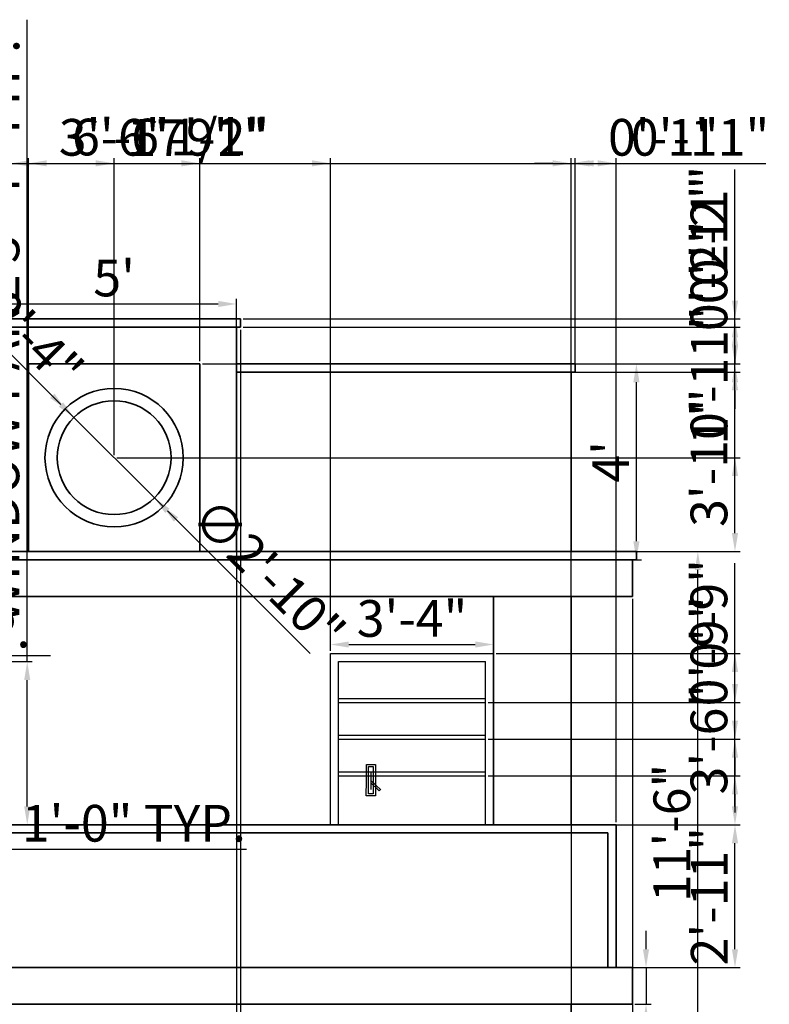
# Model space of a CAD drawing. Units: inches. Extents: x 3297 to 3846, y 520 to 959.
# Tile 5 of 5: x 3602 to 3786, y 717 to 959. Entities that reach past the tile are written whole.
import ezdxf

# ---------------------------------------------------------------- set-up
doc = ezdxf.new("R2010")
doc.units = ezdxf.units.IN
for name, color, linetype, lineweight in [('A-ANNO-DIMS', 2, 'Continuous', 18), ('A-DOOR', 4, 'Continuous', 25), ('A-ELEV', 7, 'Continuous', 35)]:
    doc.layers.add(name, color=color, linetype=linetype, lineweight=lineweight)
doc.styles.get("Standard").update_dxf_attribs({"font": 'arial.ttf'})
doc.dimstyles.new('ISO-25', dxfattribs={"dimtxt": 9, "dimasz": 4.5, "dimexe": 1.25, "dimexo": 0.625, "dimtad": 1, "dimdec": 0, "dimlunit": 3, "dimtxsty": 'Standard', "dimcen": 2.5, "dimadec": 0, "dimazin": 0, "dimtfac": 1, "dimtdec": 0, "dimtmove": 0, "dimatfit": 3, "dimfxl": 1, "dimarcsym": 0})

# ---------------------------------------------------------------- blocks, each defined once
blk = doc.blocks.new('*D2')
at = {"layer": 'A-ANNO-DIMS', "color": 0, "lineweight": -2, "transparency": 16777216}
for p, q in [((3752.69, 828.24), (3769.36, 828.24)), ((3768.11, 694.74), (3768.11, 823.74)), ((3752.69, 690.24), (3769.36, 690.24))]:
    blk.add_line(p, q, dxfattribs=at)
at = {"layer": 'A-ANNO-DIMS', "color": 0, "transparency": 16777216}
for points in [[(3767.36, 823.74), (3768.86, 823.74), (3768.11, 828.24)], [(3767.36, 694.74), (3768.86, 694.74), (3768.11, 690.24)]]:
    blk.add_solid(points, dxfattribs=at)
at = {"layer": 'Defpoints', "color": 0, "transparency": 16777216}
for p in [(3752.06, 828.24), (3768.11, 828.24), (3752.06, 690.24)]:
    blk.add_point(p, dxfattribs=at)
at = {"layer": 'A-ANNO-DIMS', "color": 0, "transparency": 16777216, "insert": (3762.89, 759.24), "char_height": 9, "attachment_point": 5, "rotation": 90}
blk.add_mtext('11\'-6"', dxfattribs=at)
blk = doc.blocks.new('*D3')
at = {"layer": 'A-ANNO-DIMS', "color": 0, "lineweight": -2, "transparency": 16777216}
for p, q in [((3738.69, 874.24), (3754.3, 874.24)), ((3753.05, 830.74), (3753.05, 869.74)), ((3738.69, 826.24), (3754.3, 826.24))]:
    blk.add_line(p, q, dxfattribs=at)
at = {"layer": 'A-ANNO-DIMS', "color": 0, "transparency": 16777216}
for points in [[(3752.3, 869.74), (3753.8, 869.74), (3753.05, 874.24)], [(3752.3, 830.74), (3753.8, 830.74), (3753.05, 826.24)]]:
    blk.add_solid(points, dxfattribs=at)
at = {"layer": 'Defpoints', "color": 0, "transparency": 16777216}
for p in [(3738.06, 874.24), (3753.05, 874.24), (3738.06, 826.24)]:
    blk.add_point(p, dxfattribs=at)
at = {"layer": 'A-ANNO-DIMS', "color": 0, "transparency": 16777216, "insert": (3747.92, 850.24), "char_height": 9, "attachment_point": 5, "rotation": 90}
blk.add_mtext("4'", dxfattribs=at)
blk = doc.blocks.new('*D13')
at = {"layer": 'A-ANNO-DIMS', "color": 0, "lineweight": -2, "transparency": 16777216}
for p, q in [((3678.06, 803.87), (3678.06, 806.69)), ((3718.06, 803.87), (3718.06, 806.69)), ((3682.56, 805.44), (3713.56, 805.44))]:
    blk.add_line(p, q, dxfattribs=at)
at = {"layer": 'A-ANNO-DIMS', "color": 0, "transparency": 16777216}
for points in [[(3682.56, 806.19), (3682.56, 804.69), (3678.06, 805.44)], [(3713.56, 806.19), (3713.56, 804.69), (3718.06, 805.44)]]:
    blk.add_solid(points, dxfattribs=at)
at = {"layer": 'Defpoints', "color": 0, "transparency": 16777216}
for p in [(3718.06, 805.44), (3678.06, 803.24), (3718.06, 803.24)]:
    blk.add_point(p, dxfattribs=at)
at = {"layer": 'A-ANNO-DIMS', "color": 0, "transparency": 16777216, "insert": (3698.06, 810.66), "char_height": 9, "attachment_point": 5}
blk.add_mtext('3\'-4"', dxfattribs=at)
blk = doc.blocks.new('*D16')
at = {"layer": 'A-ANNO-DIMS', "color": 0, "lineweight": -2, "transparency": 16777216}
for p, q in [((3595.06, 874.87), (3595.06, 890.17)), ((3599.56, 888.92), (3650.56, 888.92)), ((3655.06, 874.87), (3655.06, 890.17))]:
    blk.add_line(p, q, dxfattribs=at)
at = {"layer": 'A-ANNO-DIMS', "color": 0, "transparency": 16777216}
for points in [[(3599.56, 889.67), (3599.56, 888.17), (3595.06, 888.92)], [(3650.56, 889.67), (3650.56, 888.17), (3655.06, 888.92)]]:
    blk.add_solid(points, dxfattribs=at)
at = {"layer": 'Defpoints', "color": 0, "transparency": 16777216}
for p in [(3655.06, 888.92), (3595.06, 874.24), (3655.06, 874.24)]:
    blk.add_point(p, dxfattribs=at)
at = {"layer": 'A-ANNO-DIMS', "color": 0, "transparency": 16777216, "insert": (3625.06, 894.12), "char_height": 9, "attachment_point": 5}
blk.add_mtext("5'", dxfattribs=at)
blk = doc.blocks.new('*D17')
at = {"layer": 'A-ANNO-DIMS', "color": 0, "lineweight": -2, "transparency": 16777216}
for p, q in [((3755.4, 730.74), (3755.4, 735.24)), ((3752.69, 726.24), (3756.65, 726.24)), ((3755.4, 726.24), (3755.4, 717.24)), ((3752.69, 717.24), (3756.65, 717.24)), ((3755.4, 712.74), (3755.4, 696.65))]:
    blk.add_line(p, q, dxfattribs=at)
at = {"layer": 'A-ANNO-DIMS', "color": 0, "transparency": 16777216}
for points in [[(3754.65, 730.74), (3756.15, 730.74), (3755.4, 726.24)], [(3754.65, 712.74), (3756.15, 712.74), (3755.4, 717.24)]]:
    blk.add_solid(points, dxfattribs=at)
at = {"layer": 'Defpoints', "color": 0, "transparency": 16777216}
for p in [(3752.06, 726.24), (3752.06, 717.24), (3755.4, 717.24)]:
    blk.add_point(p, dxfattribs=at)
at = {"layer": 'A-ANNO-DIMS', "color": 0, "transparency": 16777216, "insert": (3750.18, 702.44), "char_height": 9, "attachment_point": 5, "rotation": 90}
blk.add_mtext('9"', dxfattribs=at)
blk = doc.blocks.new('*D27')
at = {"layer": 'A-ANNO-DIMS', "color": 0, "lineweight": -2, "transparency": 16777216}
for p, q in [((3603.76, 801.24), (3603.76, 958.61)), ((3598.39, 801.24), (3605.01, 801.24)), ((3603.76, 765.74), (3603.76, 796.74)), ((3598.39, 761.24), (3605.01, 761.24))]:
    blk.add_line(p, q, dxfattribs=at)
at = {"layer": 'A-ANNO-DIMS', "color": 0, "transparency": 16777216}
for points in [[(3603.01, 796.74), (3604.51, 796.74), (3603.76, 801.24)], [(3603.01, 765.74), (3604.51, 765.74), (3603.76, 761.24)]]:
    blk.add_solid(points, dxfattribs=at)
at = {"layer": 'Defpoints', "color": 0, "transparency": 16777216}
for p in [(3597.76, 801.24), (3603.76, 801.24), (3597.76, 761.24)]:
    blk.add_point(p, dxfattribs=at)
at = {"layer": 'A-ANNO-DIMS', "color": 0, "transparency": 16777216, "insert": (3598.48, 882.18), "char_height": 9, "attachment_point": 5, "rotation": 90}
blk.add_mtext('WINDOW PANE 3\'-4" TYP.', dxfattribs=at)
blk = doc.blocks.new('*D28')
at = {"layer": 'A-ANNO-DIMS', "color": 0, "lineweight": -2, "transparency": 16777216}
for p, q in [((3585.76, 760.62), (3585.76, 753.99)), ((3597.76, 760.62), (3597.76, 753.99)), ((3590.26, 755.24), (3593.26, 755.24)), ((3597.76, 755.24), (3657.53, 755.24))]:
    blk.add_line(p, q, dxfattribs=at)
at = {"layer": 'A-ANNO-DIMS', "color": 0, "transparency": 16777216}
for points in [[(3590.26, 755.99), (3590.26, 754.49), (3585.76, 755.24)], [(3593.26, 755.99), (3593.26, 754.49), (3597.76, 755.24)]]:
    blk.add_solid(points, dxfattribs=at)
at = {"layer": 'Defpoints', "color": 0, "transparency": 16777216}
for p in [(3585.76, 761.24), (3597.76, 761.24), (3597.76, 755.24)]:
    blk.add_point(p, dxfattribs=at)
at = {"layer": 'A-ANNO-DIMS', "color": 0, "transparency": 16777216, "insert": (3629.89, 760.46), "char_height": 9, "attachment_point": 5}
blk.add_mtext('1\'-0" TYP.', dxfattribs=at)
blk = doc.blocks.new('*D33')
at = {"layer": 'A-ANNO-DIMS', "color": 0, "lineweight": -2, "transparency": 16777216}
for p, q in [((3398.06, 795.31), (3398.06, 804.03)), ((3452.06, 795.31), (3452.06, 804.03)), ((3402.56, 802.78), (3447.56, 802.78)), ((3452.06, 802.78), (3609.43, 802.78))]:
    blk.add_line(p, q, dxfattribs=at)
at = {"layer": 'A-ANNO-DIMS', "color": 0, "transparency": 16777216}
for points in [[(3402.56, 803.53), (3402.56, 802.03), (3398.06, 802.78)], [(3447.56, 803.53), (3447.56, 802.03), (3452.06, 802.78)]]:
    blk.add_solid(points, dxfattribs=at)
at = {"layer": 'Defpoints', "color": 0, "transparency": 16777216}
for p in [(3452.06, 802.78), (3398.06, 794.68), (3452.06, 794.68)]:
    blk.add_point(p, dxfattribs=at)
at = {"layer": 'A-ANNO-DIMS', "color": 0, "transparency": 16777216, "insert": (3533, 808.06), "char_height": 9, "attachment_point": 5}
blk.add_mtext('WINDOW SASH 4\'-6" TYP.', dxfattribs=at)
blk = doc.blocks.new('*D35')
at = {"layer": 'A-ANNO-DIMS', "color": 0, "lineweight": -2, "transparency": 16777216}
for p, q in [((3604.06, 828.87), (3604.06, 924.64)), ((3625.06, 851.87), (3625.06, 924.64)), ((3608.56, 923.39), (3620.56, 923.39)), ((3625.06, 923.39), (3653.89, 923.39))]:
    blk.add_line(p, q, dxfattribs=at)
at = {"layer": 'A-ANNO-DIMS', "color": 0, "transparency": 16777216}
for points in [[(3608.56, 924.14), (3608.56, 922.64), (3604.06, 923.39)], [(3620.56, 924.14), (3620.56, 922.64), (3625.06, 923.39)]]:
    blk.add_solid(points, dxfattribs=at)
at = {"layer": 'Defpoints', "color": 0, "transparency": 16777216}
for p in [(3625.06, 923.39), (3625.06, 851.24), (3604.06, 828.24)]:
    blk.add_point(p, dxfattribs=at)
at = {"layer": 'A-ANNO-DIMS', "color": 0, "transparency": 16777216, "insert": (3641.73, 928.61), "char_height": 9, "attachment_point": 5}
blk.add_mtext('1\'-9"', dxfattribs=at)
blk = doc.blocks.new('*D36')
at = {"layer": 'A-ANNO-DIMS', "color": 0, "lineweight": -2, "transparency": 16777216}
for p, q in [((3777.21, 851.24), (3777.21, 887.06)), ((3625.69, 851.24), (3778.46, 851.24)), ((3777.21, 832.74), (3777.21, 846.74)), ((3604.69, 828.24), (3778.46, 828.24))]:
    blk.add_line(p, q, dxfattribs=at)
at = {"layer": 'A-ANNO-DIMS', "color": 0, "transparency": 16777216}
for points in [[(3776.46, 846.74), (3777.96, 846.74), (3777.21, 851.24)], [(3776.46, 832.74), (3777.96, 832.74), (3777.21, 828.24)]]:
    blk.add_solid(points, dxfattribs=at)
at = {"layer": 'Defpoints', "color": 0, "transparency": 16777216}
for p in [(3625.06, 851.24), (3777.21, 851.24), (3604.06, 828.24)]:
    blk.add_point(p, dxfattribs=at)
at = {"layer": 'A-ANNO-DIMS', "color": 0, "transparency": 16777216, "insert": (3772.07, 871.4), "char_height": 9, "attachment_point": 5, "rotation": 90}
blk.add_mtext('1\'-11"', dxfattribs=at)
blk = doc.blocks.new('*D37')
at = {"layer": 'A-ANNO-DIMS', "color": 0, "lineweight": -2, "transparency": 16777216}
for p, q in [((3604.06, 874.87), (3604.06, 924.64)), ((3646.06, 874.87), (3646.06, 924.64)), ((3608.56, 923.39), (3641.56, 923.39))]:
    blk.add_line(p, q, dxfattribs=at)
at = {"layer": 'A-ANNO-DIMS', "color": 0, "transparency": 16777216}
for points in [[(3608.56, 924.14), (3608.56, 922.64), (3604.06, 923.39)], [(3641.56, 924.14), (3641.56, 922.64), (3646.06, 923.39)]]:
    blk.add_solid(points, dxfattribs=at)
at = {"layer": 'Defpoints', "color": 0, "transparency": 16777216}
for p in [(3646.06, 923.39), (3604.06, 874.24), (3646.06, 874.24)]:
    blk.add_point(p, dxfattribs=at)
at = {"layer": 'A-ANNO-DIMS', "color": 0, "transparency": 16777216, "insert": (3625.06, 928.61), "char_height": 9, "attachment_point": 5}
blk.add_mtext('3\'-6"', dxfattribs=at)
blk = doc.blocks.new('*D38')
at = {"layer": 'A-ANNO-DIMS', "color": 0, "lineweight": -2, "transparency": 16777216}
for p, q in [((3646.69, 874.24), (3778.46, 874.24)), ((3777.21, 832.74), (3777.21, 869.74)), ((3646.69, 828.24), (3778.46, 828.24))]:
    blk.add_line(p, q, dxfattribs=at)
at = {"layer": 'A-ANNO-DIMS', "color": 0, "transparency": 16777216}
for points in [[(3776.46, 869.74), (3777.96, 869.74), (3777.21, 874.24)], [(3776.46, 832.74), (3777.96, 832.74), (3777.21, 828.24)]]:
    blk.add_solid(points, dxfattribs=at)
at = {"layer": 'Defpoints', "color": 0, "transparency": 16777216}
for p in [(3646.06, 874.24), (3777.21, 874.24), (3646.06, 828.24)]:
    blk.add_point(p, dxfattribs=at)
at = {"layer": 'A-ANNO-DIMS', "color": 0, "transparency": 16777216, "insert": (3771.99, 851.24), "char_height": 9, "attachment_point": 5, "rotation": 90}
blk.add_mtext('3\'-10"', dxfattribs=at)
blk = doc.blocks.new('*D39')
at = {"layer": 'A-ANNO-DIMS', "color": 0, "lineweight": -2, "transparency": 16777216}
for p, q in [((3777.21, 885.24), (3777.21, 921.91)), ((3656.69, 885.24), (3778.46, 885.24)), ((3777.21, 878.74), (3777.21, 880.74)), ((3655.69, 874.24), (3778.46, 874.24))]:
    blk.add_line(p, q, dxfattribs=at)
at = {"layer": 'A-ANNO-DIMS', "color": 0, "transparency": 16777216}
for points in [[(3776.46, 880.74), (3777.96, 880.74), (3777.21, 885.24)], [(3776.46, 878.74), (3777.96, 878.74), (3777.21, 874.24)]]:
    blk.add_solid(points, dxfattribs=at)
at = {"layer": 'Defpoints', "color": 0, "transparency": 16777216}
for p in [(3656.06, 885.24), (3777.21, 885.24), (3655.06, 874.24)]:
    blk.add_point(p, dxfattribs=at)
at = {"layer": 'A-ANNO-DIMS', "color": 0, "transparency": 16777216, "insert": (3771.99, 905.82), "char_height": 9, "attachment_point": 5, "rotation": 90}
blk.add_mtext('0\'-11"', dxfattribs=at)
blk = doc.blocks.new('*D40')
at = {"layer": 'A-ANNO-DIMS', "color": 0, "lineweight": -2, "transparency": 16777216}
for p, q in [((3777.21, 889.74), (3777.21, 919.42)), ((3656.69, 885.24), (3778.46, 885.24)), ((3777.21, 883.24), (3777.21, 885.24)), ((3656.69, 883.24), (3778.46, 883.24)), ((3777.21, 878.74), (3777.21, 874.24))]:
    blk.add_line(p, q, dxfattribs=at)
at = {"layer": 'A-ANNO-DIMS', "color": 0, "transparency": 16777216}
for points in [[(3776.46, 889.74), (3777.96, 889.74), (3777.21, 885.24)], [(3776.46, 878.74), (3777.96, 878.74), (3777.21, 883.24)]]:
    blk.add_solid(points, dxfattribs=at)
at = {"layer": 'Defpoints', "color": 0, "transparency": 16777216}
for p in [(3656.06, 885.24), (3777.21, 885.24), (3656.06, 883.24)]:
    blk.add_point(p, dxfattribs=at)
at = {"layer": 'A-ANNO-DIMS', "color": 0, "transparency": 16777216, "insert": (3771.99, 906.83), "char_height": 9, "attachment_point": 5, "rotation": 90}
blk.add_mtext('0\'-2"', dxfattribs=at)
blk = doc.blocks.new('*D41')
at = {"layer": 'A-ANNO-DIMS', "color": 0, "lineweight": -2, "transparency": 16777216}
for p, q in [((3655.06, 882.62), (3655.06, 526.84)), ((3656.06, 882.62), (3656.06, 526.84)), ((3650.56, 528.09), (3646.06, 528.09)), ((3655.06, 528.09), (3656.06, 528.09)), ((3660.56, 528.09), (3690.24, 528.09))]:
    blk.add_line(p, q, dxfattribs=at)
at = {"layer": 'A-ANNO-DIMS', "color": 0, "transparency": 16777216}
for points in [[(3650.56, 528.84), (3650.56, 527.34), (3655.06, 528.09)], [(3660.56, 528.84), (3660.56, 527.34), (3656.06, 528.09)]]:
    blk.add_solid(points, dxfattribs=at)
at = {"layer": 'Defpoints', "color": 0, "transparency": 16777216}
for p in [(3655.06, 883.24), (3656.06, 883.24), (3656.06, 528.09)]:
    blk.add_point(p, dxfattribs=at)
at = {"layer": 'A-ANNO-DIMS', "color": 0, "transparency": 16777216, "insert": (3677.65, 533.31), "char_height": 9, "attachment_point": 5}
blk.add_mtext('0\'-1"', dxfattribs=at)
blk = doc.blocks.new('*D42')
at = {"layer": 'A-ANNO-DIMS', "color": 0, "lineweight": -2, "transparency": 16777216}
for p, q in [((3777.21, 878.74), (3777.21, 908.42)), ((3655.69, 874.24), (3778.46, 874.24)), ((3777.21, 872.24), (3777.21, 874.24)), ((3655.69, 872.24), (3778.46, 872.24)), ((3777.21, 867.74), (3777.21, 863.24))]:
    blk.add_line(p, q, dxfattribs=at)
at = {"layer": 'A-ANNO-DIMS', "color": 0, "transparency": 16777216}
for points in [[(3776.46, 878.74), (3777.96, 878.74), (3777.21, 874.24)], [(3776.46, 867.74), (3777.96, 867.74), (3777.21, 872.24)]]:
    blk.add_solid(points, dxfattribs=at)
at = {"layer": 'Defpoints', "color": 0, "transparency": 16777216}
for p in [(3655.06, 874.24), (3777.21, 874.24), (3655.06, 872.24)]:
    blk.add_point(p, dxfattribs=at)
at = {"layer": 'A-ANNO-DIMS', "color": 0, "transparency": 16777216, "insert": (3771.99, 895.83), "char_height": 9, "attachment_point": 5, "rotation": 90}
blk.add_mtext('0\'-2"', dxfattribs=at)
blk = doc.blocks.new('*D44')
at = {"layer": 'A-ANNO-DIMS', "color": 0, "lineweight": -2, "transparency": 16777216}
for p, q in [((3737.06, 872.87), (3737.06, 924.64)), ((3738.06, 872.87), (3738.06, 924.64)), ((3732.56, 923.39), (3728.06, 923.39)), ((3737.06, 923.39), (3738.06, 923.39)), ((3742.56, 923.39), (3772.24, 923.39))]:
    blk.add_line(p, q, dxfattribs=at)
at = {"layer": 'A-ANNO-DIMS', "color": 0, "transparency": 16777216}
for points in [[(3732.56, 924.14), (3732.56, 922.64), (3737.06, 923.39)], [(3742.56, 924.14), (3742.56, 922.64), (3738.06, 923.39)]]:
    blk.add_solid(points, dxfattribs=at)
at = {"layer": 'Defpoints', "color": 0, "transparency": 16777216}
for p in [(3738.06, 923.39), (3737.06, 872.24), (3738.06, 872.24)]:
    blk.add_point(p, dxfattribs=at)
at = {"layer": 'A-ANNO-DIMS', "color": 0, "transparency": 16777216, "insert": (3759.65, 928.61), "char_height": 9, "attachment_point": 5}
blk.add_mtext('0\'-1"', dxfattribs=at)
blk = doc.blocks.new('*D45')
at = {"layer": 'A-ANNO-DIMS', "color": 0, "lineweight": -2, "transparency": 16777216}
for p, q in [((3737.06, 816.62), (3737.06, 526.84)), ((3752.06, 816.62), (3752.06, 526.84)), ((3741.56, 528.09), (3747.56, 528.09)), ((3752.06, 528.09), (3780.89, 528.09))]:
    blk.add_line(p, q, dxfattribs=at)
at = {"layer": 'A-ANNO-DIMS', "color": 0, "transparency": 16777216}
for points in [[(3741.56, 528.84), (3741.56, 527.34), (3737.06, 528.09)], [(3747.56, 528.84), (3747.56, 527.34), (3752.06, 528.09)]]:
    blk.add_solid(points, dxfattribs=at)
at = {"layer": 'Defpoints', "color": 0, "transparency": 16777216}
for p in [(3737.06, 817.24), (3752.06, 817.24), (3752.06, 528.09)]:
    blk.add_point(p, dxfattribs=at)
at = {"layer": 'A-ANNO-DIMS', "color": 0, "transparency": 16777216, "insert": (3768.73, 533.31), "char_height": 9, "attachment_point": 5}
blk.add_mtext('1\'-3"', dxfattribs=at)
blk = doc.blocks.new('*D67')
at = {"layer": 'A-ANNO-DIMS', "color": 0, "lineweight": -2, "transparency": 16777216}
for p, q in [((3748.69, 761.24), (3778.46, 761.24)), ((3777.21, 730.74), (3777.21, 756.74)), ((3748.69, 726.24), (3778.46, 726.24))]:
    blk.add_line(p, q, dxfattribs=at)
at = {"layer": 'A-ANNO-DIMS', "color": 0, "transparency": 16777216}
for points in [[(3776.46, 756.74), (3777.96, 756.74), (3777.21, 761.24)], [(3776.46, 730.74), (3777.96, 730.74), (3777.21, 726.24)]]:
    blk.add_solid(points, dxfattribs=at)
at = {"layer": 'Defpoints', "color": 0, "transparency": 16777216}
for p in [(3748.06, 761.24), (3777.21, 761.24), (3748.06, 726.24)]:
    blk.add_point(p, dxfattribs=at)
at = {"layer": 'A-ANNO-DIMS', "color": 0, "transparency": 16777216, "insert": (3772.07, 743.74), "char_height": 9, "attachment_point": 5, "rotation": 90}
blk.add_mtext('2\'-11"', dxfattribs=at)
blk = doc.blocks.new('*D68')
at = {"layer": 'A-ANNO-DIMS', "color": 0, "lineweight": -2, "transparency": 16777216}
for p, q in [((3737.06, 761.87), (3737.06, 924.64)), ((3748.06, 761.87), (3748.06, 924.64)), ((3741.56, 923.39), (3743.56, 923.39)), ((3748.06, 923.39), (3784.73, 923.39))]:
    blk.add_line(p, q, dxfattribs=at)
at = {"layer": 'A-ANNO-DIMS', "color": 0, "transparency": 16777216}
for points in [[(3741.56, 924.14), (3741.56, 922.64), (3737.06, 923.39)], [(3743.56, 924.14), (3743.56, 922.64), (3748.06, 923.39)]]:
    blk.add_solid(points, dxfattribs=at)
at = {"layer": 'Defpoints', "color": 0, "transparency": 16777216}
for p in [(3748.06, 923.39), (3737.06, 761.24), (3748.06, 761.24)]:
    blk.add_point(p, dxfattribs=at)
at = {"layer": 'A-ANNO-DIMS', "color": 0, "transparency": 16777216, "insert": (3768.65, 928.61), "char_height": 9, "attachment_point": 5}
blk.add_mtext('0\'-11"', dxfattribs=at)
blk = doc.blocks.new('*D69')
at = {"layer": 'A-ANNO-DIMS', "color": 0, "lineweight": -2, "transparency": 16777216}
for p, q in [((3543.06, 759.87), (3543.06, 924.64)), ((3748.06, 761.87), (3748.06, 924.64)), ((3547.56, 923.39), (3743.56, 923.39))]:
    blk.add_line(p, q, dxfattribs=at)
at = {"layer": 'A-ANNO-DIMS', "color": 0, "transparency": 16777216}
for points in [[(3547.56, 924.14), (3547.56, 922.64), (3543.06, 923.39)], [(3743.56, 924.14), (3743.56, 922.64), (3748.06, 923.39)]]:
    blk.add_solid(points, dxfattribs=at)
at = {"layer": 'Defpoints', "color": 0, "transparency": 16777216}
for p in [(3748.06, 923.39), (3748.06, 761.24), (3543.06, 759.24)]:
    blk.add_point(p, dxfattribs=at)
at = {"layer": 'A-ANNO-DIMS', "color": 0, "transparency": 16777216, "insert": (3645.56, 928.53), "char_height": 9, "attachment_point": 5}
blk.add_mtext('17\'-1"', dxfattribs=at)
blk = doc.blocks.new('*D70')
at = {"layer": 'A-ANNO-DIMS', "color": 0, "lineweight": -2, "transparency": 16777216}
for p, q in [((3555.76, 760.62), (3555.76, 526.84)), ((3543.06, 758.62), (3543.06, 526.84)), ((3547.56, 528.09), (3551.26, 528.09)), ((3555.76, 528.09), (3605.56, 528.09))]:
    blk.add_line(p, q, dxfattribs=at)
at = {"layer": 'A-ANNO-DIMS', "color": 0, "transparency": 16777216}
for points in [[(3547.56, 528.84), (3547.56, 527.34), (3543.06, 528.09)], [(3551.26, 528.84), (3551.26, 527.34), (3555.76, 528.09)]]:
    blk.add_solid(points, dxfattribs=at)
at = {"layer": 'Defpoints', "color": 0, "transparency": 16777216}
for p in [(3555.76, 761.24), (3543.06, 759.24), (3555.76, 528.09)]:
    blk.add_point(p, dxfattribs=at)
at = {"layer": 'A-ANNO-DIMS', "color": 0, "transparency": 16777216, "insert": (3582.91, 533.37), "char_height": 9, "attachment_point": 5}
blk.add_mtext('1\'-0 1/2"', dxfattribs=at)
blk = doc.blocks.new('*D73')
at = {"layer": 'A-ANNO-DIMS', "color": 0, "lineweight": -2, "transparency": 16777216}
for p, q in [((3599.76, 803.87), (3599.76, 924.64)), ((3678.06, 803.87), (3678.06, 924.64)), ((3604.26, 923.39), (3673.56, 923.39))]:
    blk.add_line(p, q, dxfattribs=at)
at = {"layer": 'A-ANNO-DIMS', "color": 0, "transparency": 16777216}
for points in [[(3604.26, 924.14), (3604.26, 922.64), (3599.76, 923.39)], [(3673.56, 924.14), (3673.56, 922.64), (3678.06, 923.39)]]:
    blk.add_solid(points, dxfattribs=at)
at = {"layer": 'Defpoints', "color": 0, "transparency": 16777216}
for p in [(3678.06, 923.39), (3599.76, 803.24), (3678.06, 803.24)]:
    blk.add_point(p, dxfattribs=at)
at = {"layer": 'A-ANNO-DIMS', "color": 0, "transparency": 16777216, "insert": (3638.91, 928.67), "char_height": 9, "attachment_point": 5}
blk.add_mtext('6\'-6 1/2"', dxfattribs=at)
blk = doc.blocks.new('*D74')
at = {"layer": 'A-ANNO-DIMS', "color": 0, "lineweight": -2, "transparency": 16777216}
for p, q in [((3718.69, 803.24), (3778.46, 803.24)), ((3777.21, 765.74), (3777.21, 798.74)), ((3718.69, 761.24), (3778.46, 761.24))]:
    blk.add_line(p, q, dxfattribs=at)
at = {"layer": 'A-ANNO-DIMS', "color": 0, "transparency": 16777216}
for points in [[(3776.46, 798.74), (3777.96, 798.74), (3777.21, 803.24)], [(3776.46, 765.74), (3777.96, 765.74), (3777.21, 761.24)]]:
    blk.add_solid(points, dxfattribs=at)
at = {"layer": 'Defpoints', "color": 0, "transparency": 16777216}
for p in [(3718.06, 803.24), (3777.21, 803.24), (3718.06, 761.24)]:
    blk.add_point(p, dxfattribs=at)
at = {"layer": 'A-ANNO-DIMS', "color": 0, "transparency": 16777216, "insert": (3771.99, 782.24), "char_height": 9, "attachment_point": 5, "rotation": 90}
blk.add_mtext('3\'-6"', dxfattribs=at)
blk = doc.blocks.new('*D75')
at = {"layer": 'A-ANNO-DIMS', "color": 0, "lineweight": -2, "transparency": 16777216}
for p, q in [((3777.21, 786.74), (3777.21, 816.42)), ((3716.69, 782.24), (3778.46, 782.24)), ((3777.21, 773.24), (3777.21, 782.24)), ((3716.69, 773.24), (3778.46, 773.24)), ((3777.21, 768.74), (3777.21, 764.24))]:
    blk.add_line(p, q, dxfattribs=at)
at = {"layer": 'A-ANNO-DIMS', "color": 0, "transparency": 16777216}
for points in [[(3776.46, 786.74), (3777.96, 786.74), (3777.21, 782.24)], [(3776.46, 768.74), (3777.96, 768.74), (3777.21, 773.24)]]:
    blk.add_solid(points, dxfattribs=at)
at = {"layer": 'Defpoints', "color": 0, "transparency": 16777216}
for p in [(3716.06, 782.24), (3777.21, 782.24), (3716.06, 773.24)]:
    blk.add_point(p, dxfattribs=at)
at = {"layer": 'A-ANNO-DIMS', "color": 0, "transparency": 16777216, "insert": (3771.99, 803.83), "char_height": 9, "attachment_point": 5, "rotation": 90}
blk.add_mtext('0\'-9"', dxfattribs=at)
blk = doc.blocks.new('*D76')
at = {"layer": 'A-ANNO-DIMS', "color": 0, "lineweight": -2, "transparency": 16777216}
for p, q in [((3777.21, 795.74), (3777.21, 825.42)), ((3716.69, 791.24), (3778.46, 791.24)), ((3777.21, 782.24), (3777.21, 791.24)), ((3716.69, 782.24), (3778.46, 782.24)), ((3777.21, 777.74), (3777.21, 773.24))]:
    blk.add_line(p, q, dxfattribs=at)
at = {"layer": 'A-ANNO-DIMS', "color": 0, "transparency": 16777216}
for points in [[(3776.46, 795.74), (3777.96, 795.74), (3777.21, 791.24)], [(3776.46, 777.74), (3777.96, 777.74), (3777.21, 782.24)]]:
    blk.add_solid(points, dxfattribs=at)
at = {"layer": 'Defpoints', "color": 0, "transparency": 16777216}
for p in [(3716.06, 791.24), (3777.21, 791.24), (3716.06, 782.24)]:
    blk.add_point(p, dxfattribs=at)
at = {"layer": 'A-ANNO-DIMS', "color": 0, "transparency": 16777216, "insert": (3771.99, 812.83), "char_height": 9, "attachment_point": 5, "rotation": 90}
blk.add_mtext('0\'-9"', dxfattribs=at)
blk = doc.blocks.new('*D81')
at = {"layer": 'A-ANNO-DIMS', "color": 0, "lineweight": -2, "transparency": 16777216}
for p, q in [((3609.9, 866.4), (3606.71, 869.59)), ((3613.08, 863.22), (3637.05, 839.26)), ((3673.09, 803.23), (3640.23, 836.08))]:
    blk.add_line(p, q, dxfattribs=at)
at = {"layer": 'A-ANNO-DIMS', "color": 0, "transparency": 16777216}
for points in [[(3610.43, 866.93), (3609.37, 865.87), (3613.08, 863.22)], [(3640.76, 836.61), (3639.7, 835.55), (3637.05, 839.26)]]:
    blk.add_solid(points, dxfattribs=at)
at = {"layer": 'Defpoints', "color": 0, "transparency": 16777216}
for p in [(3613.08, 863.22), (3637.05, 839.26)]:
    blk.add_point(p, dxfattribs=at)
at = {"layer": 'A-ANNO-DIMS', "color": 0, "transparency": 16777216, "insert": (3662.12, 821.93), "char_height": 9, "attachment_point": 5, "rotation": 315.0098}
blk.add_mtext('∅2\'-10"', dxfattribs=at)
blk = doc.blocks.new('*D82')
at = {"layer": 'A-ANNO-DIMS', "color": 0, "lineweight": -2, "transparency": 16777216}
for p, q in [((3584.1, 892.18), (3612.02, 864.28)), ((3634.93, 841.38), (3615.2, 861.1)), ((3638.11, 838.2), (3641.3, 835.02))]:
    blk.add_line(p, q, dxfattribs=at)
at = {"layer": 'A-ANNO-DIMS', "color": 0, "transparency": 16777216}
for points in [[(3612.55, 864.81), (3611.49, 863.75), (3615.2, 861.1)], [(3638.64, 838.73), (3637.58, 837.67), (3634.93, 841.38)]]:
    blk.add_solid(points, dxfattribs=at)
at = {"layer": 'Defpoints', "color": 0, "transparency": 16777216}
for p in [(3615.2, 861.1), (3634.93, 841.38)]:
    blk.add_point(p, dxfattribs=at)
at = {"layer": 'A-ANNO-DIMS', "color": 0, "transparency": 16777216, "insert": (3600.34, 883.69), "char_height": 9, "attachment_point": 5, "rotation": 315.0171}
blk.add_mtext('∅2\'-4"', dxfattribs=at)

msp = doc.modelspace()

# ---------------------------------------------------------------- linework, layer by layer
at = {"layer": 'A-DOOR'}
for p, q in [((3678.06, 803.24), (3718.06, 803.24)), ((3678.06, 761.24), (3678.06, 803.24)), ((3680.06, 801.24), (3716.06, 801.24)), ((3680.06, 761.24), (3680.06, 801.24)), ((3716.06, 761.24), (3716.06, 801.24)), ((3680.06, 792.24), (3716.06, 792.24)), ((3680.06, 791.24), (3716.06, 791.24)), ((3680.06, 783.24), (3686.91, 783.24)), ((3680.06, 783.24), (3716.06, 783.24)), ((3680.06, 782.24), (3686.91, 782.24)), ((3680.06, 782.24), (3716.06, 782.24)), ((3686.91, 772.06), (3686.91, 776)), ((3686.91, 776), (3689.07, 776)), ((3687.41, 772.06), (3687.41, 775.5)), ((3687.41, 775.5), (3688.57, 775.5)), ((3688.57, 775.5), (3688.57, 768.86)), ((3689.07, 776), (3689.07, 768.36)), ((3680.06, 774.24), (3716.06, 774.24)), ((3680.06, 773.24), (3716.06, 773.24)), ((3687.99, 774.33), (3687.99, 769.92)), ((3686.85, 768.36), (3686.91, 772.06)), ((3687.36, 768.86), (3687.41, 772.05)), ((3687.99, 772.13), (3690.38, 769.83)), ((3690.03, 769.54), (3687.99, 771.57)), ((3690.34, 769.86), (3688.57, 771.57)), ((3689.07, 768.36), (3686.85, 768.36)), ((3688.57, 768.86), (3687.36, 768.86)), ((3690.34, 769.86), (3690.03, 769.54)), ((3690.38, 769.83), (3690.34, 769.86))]:
    msp.add_line(p, q, dxfattribs=at)
at = {"layer": 'A-ELEV'}
for p, q in [((3594.06, 885.24), (3656.06, 885.24)), ((3656.06, 885.24), (3656.06, 883.24)), ((3594.06, 883.24), (3656.06, 883.24)), ((3655.06, 883.24), (3655.06, 828.24)), ((3604.06, 874.24), (3646.06, 874.24)), ((3604.06, 874.24), (3604.06, 828.24)), ((3646.06, 874.24), (3646.06, 828.24)), ((3655.06, 874.24), (3738.06, 874.24)), ((3738.06, 874.24), (3738.06, 872.24)), ((3655.06, 872.24), (3738.06, 872.24)), ((3737.06, 828.24), (3737.06, 872.24)), ((3512.06, 828.24), (3753.06, 828.24)), ((3753.06, 828.24), (3753.06, 826.24)), ((3512.06, 826.24), (3753.06, 826.24)), ((3752.06, 826.24), (3752.06, 817.24)), ((3521.06, 817.24), (3752.06, 817.24)), ((3718.06, 761.24), (3718.06, 817.24)), ((3737.06, 761.24), (3737.06, 817.24)), ((3543.06, 761.24), (3748.06, 761.24)), ((3748.06, 726.24), (3748.06, 761.24)), ((3543.06, 759.24), (3746.06, 759.24)), ((3746.06, 726.24), (3746.06, 759.24)), ((3521.06, 726.24), (3752.06, 726.24)), ((3752.06, 717.24), (3752.06, 726.24)), ((3512.06, 717.24), (3752.06, 717.24)), ((3737.06, 690.24), (3737.06, 717.24))]:
    msp.add_line(p, q, dxfattribs=at)
for radius in [16.95, 13.95]:
    msp.add_circle((3625.06, 851.24), radius, dxfattribs=at)

# ---------------------------------------------------------------- dimensions: what is measured, and where the dimension line sits
at = {"layer": 'A-ANNO-DIMS'}
dim = msp.add_linear_dim(base=(3603.76, 801.24), p1=(3597.76, 761.24), p2=(3597.76, 801.24), angle=90, text='WINDOW PANE <> TYP.', dimstyle='ISO-25', override={"dimdec": 1, "dimrnd": 0, "dimzin": 1, "dimlunit": 4, "dimfrac": 2}, dxfattribs=at)
dim.commit()
dim.dimension.update_dxf_attribs({"geometry": '*D27', "text_midpoint": (3598.48, 882.18)})
for base, p1, p2, override, picture, middle in [((3678.06, 923.39), (3599.76, 803.24), (3678.06, 803.24), {"dimdec": 1, "dimlfac": 1, "dimrnd": 0, "dimzin": 1, "dimdsep": 46, "dimlunit": 4, "dimfrac": 2}, '*D73', (3638.91, 928.67)), ((3748.06, 923.39), (3543.06, 759.24), (3748.06, 761.24), {"dimdec": 1, "dimlfac": 1, "dimrnd": 0, "dimzin": 1, "dimdsep": 46, "dimlunit": 4, "dimfrac": 2}, '*D69', (3645.56, 928.53)), ((3646.06, 923.39), (3604.06, 874.24), (3646.06, 874.24), {"dimdec": 1, "dimlfac": 1, "dimrnd": 0, "dimzin": 1, "dimdsep": 46, "dimlunit": 4, "dimfrac": 2}, '*D37', (3625.06, 928.61)), ((3625.06, 923.39), (3604.06, 828.24), (3625.06, 851.24), {"dimdec": 1, "dimlfac": 1, "dimrnd": 0, "dimzin": 1, "dimdsep": 46, "dimlunit": 4, "dimfrac": 2}, '*D35', (3641.73, 928.61)), ((3738.06, 923.39), (3737.06, 872.24), (3738.06, 872.24), {"dimdec": 1, "dimlfac": 1, "dimrnd": 0, "dimzin": 1, "dimdsep": 46, "dimlunit": 4, "dimfrac": 2}, '*D44', (3759.65, 928.61)), ((3748.06, 923.39), (3737.06, 761.24), (3748.06, 761.24), {"dimdec": 1, "dimlfac": 1, "dimrnd": 0, "dimzin": 1, "dimdsep": 46, "dimlunit": 4, "dimfrac": 2}, '*D68', (3768.65, 928.61)), ((3655.06, 888.92), (3595.06, 874.24), (3655.06, 874.24), {"dimclrd": 0, "dimclre": 0, "dimclrt": 0}, '*D16', (3625.06, 894.12)), ((3656.06, 528.09), (3655.06, 883.24), (3656.06, 883.24), {"dimdec": 1, "dimlfac": 1, "dimrnd": 0, "dimzin": 1, "dimdsep": 46, "dimlunit": 4, "dimfrac": 2}, '*D41', (3677.65, 533.31)), ((3718.06, 805.44), (3678.06, 803.24), (3718.06, 803.24), {"dimclrd": 0, "dimclre": 0, "dimclrt": 0}, '*D13', (3698.06, 810.66)), ((3752.06, 528.09), (3737.06, 817.24), (3752.06, 817.24), {"dimdec": 1, "dimlfac": 1, "dimrnd": 0, "dimzin": 1, "dimdsep": 46, "dimlunit": 4, "dimfrac": 2}, '*D45', (3768.73, 533.31)), ((3555.76, 528.09), (3543.06, 759.24), (3555.76, 761.24), {"dimdec": 1, "dimlfac": 1, "dimrnd": 0, "dimzin": 1, "dimdsep": 46, "dimlunit": 4, "dimfrac": 2}, '*D70', (3582.91, 533.37))]:
    dim = msp.add_linear_dim(base=base, p1=p1, p2=p2, dimstyle='ISO-25', override=override, dxfattribs=at)
    dim.commit()
    dim.dimension.update_dxf_attribs({"geometry": picture, "text_midpoint": middle})
for base, p1, p2, override, picture, middle in [((3777.21, 885.24), (3655.06, 874.24), (3656.06, 885.24), {"dimdec": 1, "dimlfac": 1, "dimrnd": 0, "dimzin": 1, "dimdsep": 46, "dimlunit": 4, "dimfrac": 2}, '*D39', (3771.99, 905.82)), ((3777.21, 885.24), (3656.06, 883.24), (3656.06, 885.24), {"dimdec": 1, "dimlfac": 1, "dimrnd": 0, "dimzin": 1, "dimdsep": 46, "dimlunit": 4, "dimfrac": 2}, '*D40', (3771.99, 906.83)), ((3777.21, 874.24), (3655.06, 872.24), (3655.06, 874.24), {"dimdec": 1, "dimlfac": 1, "dimrnd": 0, "dimzin": 1, "dimdsep": 46, "dimlunit": 4, "dimfrac": 2}, '*D42', (3771.99, 895.83)), ((3777.21, 851.24), (3604.06, 828.24), (3625.06, 851.24), {"dimdec": 1, "dimlfac": 1, "dimrnd": 0, "dimzin": 1, "dimdsep": 46, "dimlunit": 4, "dimfrac": 2}, '*D36', (3772.07, 871.4)), ((3777.21, 874.24), (3646.06, 828.24), (3646.06, 874.24), {"dimdec": 1, "dimlfac": 1, "dimrnd": 0, "dimzin": 1, "dimdsep": 46, "dimlunit": 4, "dimfrac": 2}, '*D38', (3771.99, 851.24)), ((3753.05, 874.24), (3738.06, 826.24), (3738.06, 874.24), {"dimclrd": 0, "dimclre": 0, "dimclrt": 0}, '*D3', (3747.92, 850.24)), ((3768.11, 828.24), (3752.06, 690.24), (3752.06, 828.24), {"dimclrd": 0, "dimclre": 0, "dimclrt": 0}, '*D2', (3762.89, 759.24)), ((3777.21, 791.24), (3716.06, 782.24), (3716.06, 791.24), {"dimdec": 1, "dimlfac": 1, "dimrnd": 0, "dimzin": 1, "dimdsep": 46, "dimlunit": 4, "dimfrac": 2}, '*D76', (3771.99, 812.83)), ((3777.21, 782.24), (3716.06, 773.24), (3716.06, 782.24), {"dimdec": 1, "dimlfac": 1, "dimrnd": 0, "dimzin": 1, "dimdsep": 46, "dimlunit": 4, "dimfrac": 2}, '*D75', (3771.99, 803.83)), ((3777.21, 803.24), (3718.06, 761.24), (3718.06, 803.24), {"dimdec": 1, "dimlfac": 1, "dimrnd": 0, "dimzin": 1, "dimdsep": 46, "dimlunit": 4, "dimfrac": 2}, '*D74', (3771.99, 782.24)), ((3777.21, 761.24), (3748.06, 726.24), (3748.06, 761.24), {"dimdec": 1, "dimlfac": 1, "dimrnd": 0, "dimzin": 1, "dimdsep": 46, "dimlunit": 4, "dimfrac": 2}, '*D67', (3772.07, 743.74)), ((3755.4, 717.24), (3752.06, 726.24), (3752.06, 717.24), {"dimclrd": 0, "dimclre": 0, "dimclrt": 0}, '*D17', (3750.18, 702.44))]:
    dim = msp.add_linear_dim(base=base, p1=p1, p2=p2, angle=90, dimstyle='ISO-25', override=override, dxfattribs=at)
    dim.commit()
    dim.dimension.update_dxf_attribs({"geometry": picture, "text_midpoint": middle})
for p1, p2, picture, middle in [((3634.93, 841.38), (3615.2, 861.1), '*D82', (3596.47, 879.82)), ((3613.08, 863.22), (3637.05, 839.26), '*D81', (3658.25, 818.06))]:
    dim = msp.add_diameter_dim_2p(p1=p1, p2=p2, dimstyle='ISO-25', override={"dimdec": 1, "dimlfac": 1, "dimrnd": 0, "dimzin": 1, "dimdsep": 46, "dimlunit": 4, "dimfrac": 2}, dxfattribs=at)
    dim.commit()
    dim.dimension.update_dxf_attribs({"geometry": picture, "text_midpoint": middle, "dimtype": 163})
for base, p1, p2, text, picture, middle in [((3452.06, 802.78), (3398.06, 794.68), (3452.06, 794.68), 'WINDOW SASH <> TYP.', '*D33', (3533, 808.06)), ((3597.76, 755.24), (3585.76, 761.24), (3597.76, 761.24), '<> TYP.', '*D28', (3629.89, 760.46))]:
    dim = msp.add_linear_dim(base=base, p1=p1, p2=p2, text=text, dimstyle='ISO-25', override={"dimdec": 1, "dimrnd": 0, "dimzin": 1, "dimlunit": 4, "dimfrac": 2}, dxfattribs=at)
    dim.commit()
    dim.dimension.update_dxf_attribs({"geometry": picture, "text_midpoint": middle})

doc.saveas('drawing.dxf')
